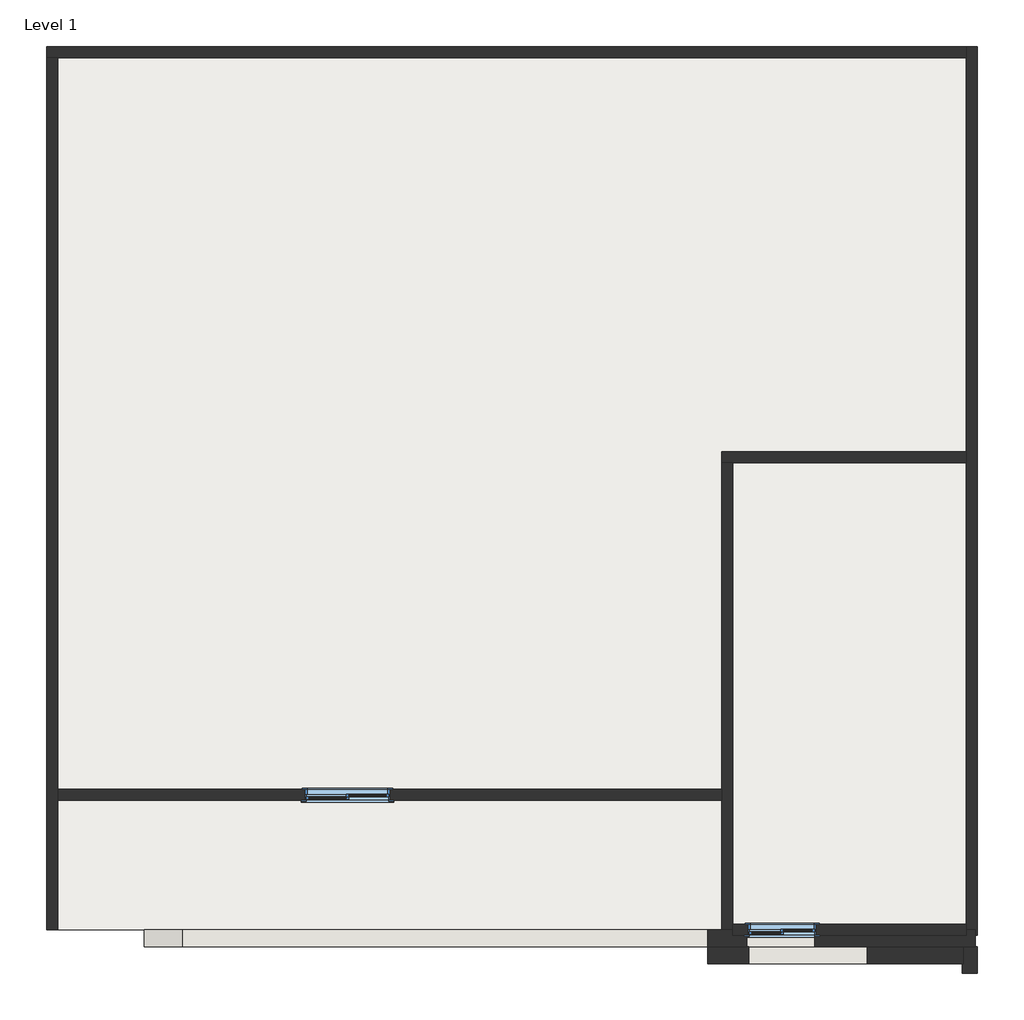
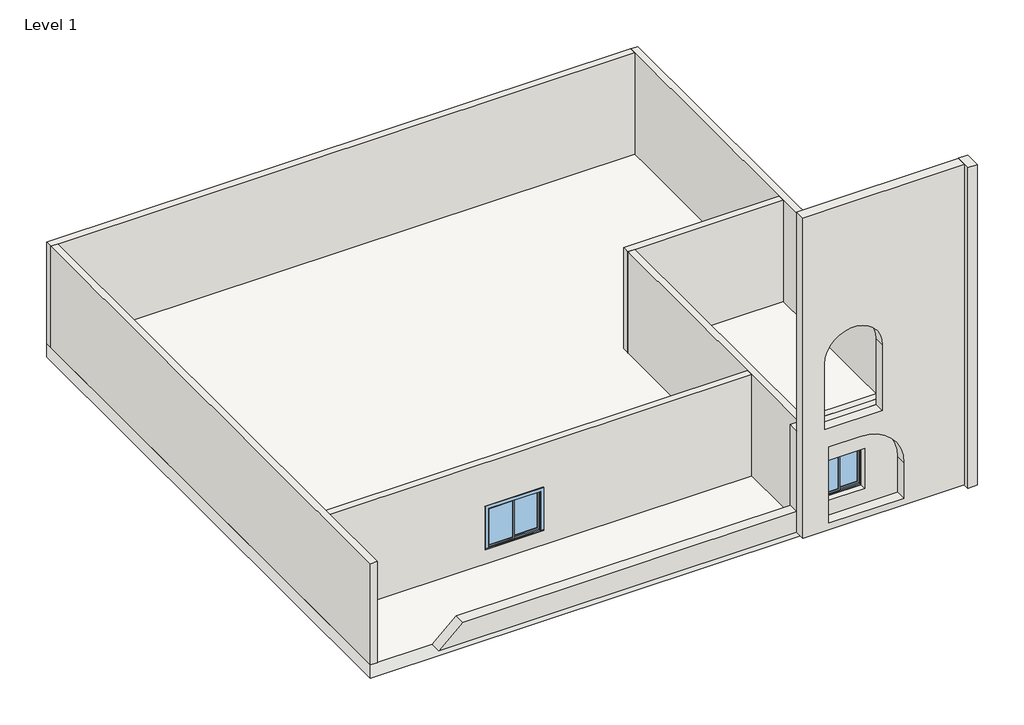
# One storey: 10 walls, 2 windows, 1 slab.
"""IFC4 building model written with IfcOpenShell, lengths in millimetres."""

from ifc_helpers import new_model, si_unit, frame, origin, place, context, project, spatial, polyline, outline, extrude, faceted_brep, transform, mapped, element, save
from components import walls_3_walls_3_95cfad7e, walls_4_walls_4_52940900, walls_6_walls_6_1b60e08d, window_deda82dd, window_c4d7a2b1

model = new_model("IFC4")

# Units and contexts
model_context = context("Model", 3, world=origin())
ifc_project = project(units=[si_unit("LENGTHUNIT", "METRE", prefix="MILLI")], contexts=[model_context])

# Site, building, storey
site = spatial("IfcSite", under=ifc_project)
building = spatial("IfcBuilding", under=site)
storey = spatial("IfcBuildingStorey", under=building, Name="Level 1", Elevation=3048.0)

# Slab
placement = place(None, origin())
element("IfcSlab", 1, ObjectType="Generic Floor - 400mm", at=placement, inside=storey, context=model_context, shape_type="SweptSolid", body=[
    extrude(outline(polyline([(-9031.8352527, 15360.4148445), (7778.3159626, 15360.4148445), (7778.3159626, -589.1851555), (-9031.8352527, -589.1851555), (-9031.8352527, 15360.4148445)])), frame((0.0, 0.0, 2648.0), z_axis=(0.0, 0.0, 1.0), x_axis=(1.0, 0.0, 0.0)), (0.0, 0.0, 1.0), 400.0),
])

# Walls
element("IfcWall", 2, ObjectType="Generic - 9\"", at=placement, inside=storey, context=model_context, shape_type="Brep", body=[
    faceted_brep([(-9031.8352527, 15160.4148445, 3048.0), (-8831.8352527, 15160.4148445, 3048.0), (7578.3159626, 15160.4148445, 3048.0), (7578.3159626, 15160.4148445, 6096.0), (-8831.8352527, 15160.4148445, 6096.0), (-9031.8352527, 15160.4148445, 6096.0), (-9031.8352527, 15360.4148445, 3048.0), (-9031.8352527, 15360.4148445, 6096.0), (7578.3159626, 15360.4148445, 6096.0), (7578.3159626, 15360.4148445, 3048.0)], [[[0, 1, 2, 3, 4, 5]], [[6, 7, 8, 9]], [[2, 1, 0, 6, 9]], [[5, 4, 3, 8, 7]], [[0, 5, 7, 6]], [[3, 2, 9, 8]]]),
])
element("IfcWall", 3, ObjectType="Generic - 9\"", at=placement, inside=storey, context=model_context, shape_type="Brep", body=[
    faceted_brep([(-8831.8352527, -589.1851555, 3048.0), (-8831.8352527, 1749.2148445, 3048.0), (-8831.8352527, 1949.2148445, 3048.0), (-8831.8352527, 15160.4148445, 3048.0), (-8831.8352527, 15160.4148445, 6096.0), (-8831.8352527, 1949.2148445, 6096.0), (-8831.8352527, 1749.2148445, 6096.0), (-8831.8352527, -589.1851555, 6096.0), (-9031.8352527, -589.1851555, 3048.0), (-9031.8352527, -589.1851555, 6096.0), (-9031.8352527, 15160.4148445, 6096.0), (-9031.8352527, 15160.4148445, 3048.0)], [[[0, 1, 2, 3, 4, 5, 6, 7]], [[8, 9, 10, 11]], [[3, 2, 1, 0, 8, 11]], [[7, 6, 5, 4, 10, 9]], [[0, 7, 9, 8]], [[4, 3, 11, 10]]]),
])
element("IfcWall", 4, ObjectType="Generic - 9\"", at=placement, inside=storey, context=model_context, shape_type="Brep", body=[
    faceted_brep([(7578.3159626, 15360.4148445, 3048.0), (7578.3159626, 15160.4148445, 3048.0), (7578.3159626, 8045.2148445, 3048.0), (7578.3159626, 7845.2148445, 3048.0), (7578.3159626, -489.1851555, 3048.0), (7578.3159626, -589.1851555, 3048.0), (7578.3159626, -689.1851555, 3048.0), (7578.3159626, -689.1851555, 6096.0), (7578.3159626, -489.1851555, 6096.0), (7578.3159626, 7845.2148445, 6096.0), (7578.3159626, 8045.2148445, 6096.0), (7578.3159626, 15160.4148445, 6096.0), (7578.3159626, 15360.4148445, 6096.0), (7778.3159626, 15360.4148445, 3048.0), (7778.3159626, 15360.4148445, 6096.0), (7778.3159626, -689.1851555, 6096.0), (7778.3159626, -689.1851555, 3048.0), (7778.3159626, -589.1851555, 3048.0), (7778.3159626, -489.1851555, 3048.0)], [[[0, 1, 2, 3, 4, 5, 6, 7, 8, 9, 10, 11, 12]], [[13, 14, 15, 16, 17, 18]], [[6, 5, 4, 3, 2, 1, 0, 13, 18, 17, 16]], [[12, 11, 10, 9, 8, 7, 15, 14]], [[0, 12, 14, 13]], [[7, 6, 16, 15]]]),
])
element("IfcWall", 5, ObjectType="Generic - 9\"", at=placement, inside=storey, context=model_context, shape_type="Brep", body=[
    faceted_brep([(3160.1647473, 7845.2148445, 3048.0), (3360.1647473, 7845.2148445, 3048.0), (7578.3159626, 7845.2148445, 3048.0), (7578.3159626, 7845.2148445, 6096.0), (3360.1647473, 7845.2148445, 6096.0), (3160.1647473, 7845.2148445, 6096.0), (3160.1647473, 8045.2148445, 3048.0), (3160.1647473, 8045.2148445, 6096.0), (7578.3159626, 8045.2148445, 6096.0), (7578.3159626, 8045.2148445, 3048.0)], [[[0, 1, 2, 3, 4, 5]], [[6, 7, 8, 9]], [[2, 1, 0, 6, 9]], [[5, 4, 3, 8, 7]], [[0, 5, 7, 6]], [[3, 2, 9, 8]]]),
])
element("IfcWall", 6, ObjectType="Generic - 9\"", at=placement, inside=storey, context=model_context, shape_type="Brep", body=[
    faceted_brep([(3360.1647473, -689.1851555, 3048.0), (3360.1647473, -489.1851555, 3048.0), (3360.1647473, 7845.2148445, 3048.0), (3360.1647473, 7845.2148445, 6096.0), (3360.1647473, -489.1851555, 6096.0), (3360.1647473, -689.1851555, 6096.0), (3160.1647473, -689.1851555, 3048.0), (3160.1647473, -689.1851555, 6096.0), (3160.1647473, 1749.2148445, 6096.0), (3160.1647473, 1949.2148445, 6096.0), (3160.1647473, 7845.2148445, 6096.0), (3160.1647473, 7845.2148445, 3048.0), (3160.1647473, 1949.2148445, 3048.0), (3160.1647473, 1749.2148445, 3048.0)], [[[0, 1, 2, 3, 4, 5]], [[6, 7, 8, 9, 10, 11, 12, 13]], [[2, 1, 0, 6, 13, 12, 11]], [[5, 4, 3, 10, 9, 8, 7]], [[3, 2, 11, 10]], [[0, 5, 7, 6]]]),
])
element("IfcWall", 7, ObjectType="Generic - 9\"", at=placement, inside=storey, context=model_context, shape_type="SweptSolid", body=[
    extrude(outline(polyline([(3048.0, 3160.1647473), (6096.0, 3160.1647473), (6096.0, -8831.8352527), (3048.0, -8831.8352527), (3048.0, 3160.1647473)]), holes=[polyline([(4724.4, -4359.8352527), (4724.4, -2835.8352527), (3505.2, -2835.8352527), (3505.2, -4359.8352527), (4724.4, -4359.8352527)])]), frame((0.0, 1749.2148445, 0.0), z_axis=(0.0, 1.0, 0.0), x_axis=(0.0, 0.0, 1.0)), (0.0, 0.0, 1.0), 200.0),
])
element("IfcWall", 8, ObjectType="Generic - 9\"", at=placement, inside=storey, context=model_context, shape_type="SweptSolid", body=[
    extrude(outline(polyline([(3048.0, 3360.1647473), (3048.0, 7578.3159626), (6096.0, 7578.3159626), (6096.0, 3360.1647473), (3048.0, 3360.1647473)]), holes=[polyline([(4906.7280725, 3641.1647473), (4906.7280725, 4860.3647473), (3687.5280725, 4860.3647473), (3687.5280725, 3641.1647473), (4906.7280725, 3641.1647473)])]), frame((0.0, -689.1851555, 0.0), z_axis=(0.0, 1.0, 0.0), x_axis=(0.0, 0.0, 1.0)), (0.0, 0.0, 1.0), 200.0),
])
walls_3_walls_3_shape = walls_3_walls_3_95cfad7e(model_context)
element("IfcWall", 9, ObjectType="Walls 3 : Walls 3", at=placement, inside=storey, context=model_context, shape_type="MappedRepresentation", body=[
    mapped(walls_3_walls_3_shape, transform((0.0, 0.0, 0.0), x_axis=(1.0, 0.0, 0.0), y_axis=(0.0, 1.0, 0.0), z_axis=(0.0, 0.0, 1.0))),
])
walls_4_walls_4_shape = walls_4_walls_4_52940900(model_context)
element("IfcWall", 10, ObjectType="Walls 4 : Walls 4", at=placement, inside=storey, context=model_context, shape_type="MappedRepresentation", body=[
    mapped(walls_4_walls_4_shape, transform((0.0, 0.0, 0.0), x_axis=(1.0, 0.0, 0.0), y_axis=(0.0, 1.0, 0.0), z_axis=(0.0, 0.0, 1.0))),
])
walls_6_walls_6_shape = walls_6_walls_6_1b60e08d(model_context)
element("IfcWall", 11, ObjectType="Walls 6 : Walls 6", at=placement, inside=storey, context=model_context, shape_type="MappedRepresentation", body=[
    mapped(walls_6_walls_6_shape, transform((0.0, 0.0, 0.0), x_axis=(1.0, 0.0, 0.0), y_axis=(0.0, 1.0, 0.0), z_axis=(0.0, 0.0, 1.0))),
])

# Windows
window_shape = window_deda82dd(model_context)
element("IfcWindow", 12, ObjectType="Slider with Trim : 48\" x 48\"", at=placement, inside=storey, context=model_context, shape_type="MappedRepresentation", body=[
    mapped(window_shape, transform((4250.7647473, -589.1851555, 2773.1280725), x_axis=(-1.0, 0.0, 0.0), y_axis=(0.0, -1.0, 0.0), z_axis=(0.0, 0.0, 1.0))),
])
window_2_shape = window_c4d7a2b1(model_context)
element("IfcWindow", 13, ObjectType="Slider with Trim : 60\" x 48\"", at=placement, inside=storey, context=model_context, shape_type="MappedRepresentation", body=[
    mapped(window_2_shape, transform((-3597.8352527, 1849.2148445, 2590.8), x_axis=(-1.0, 0.0, 0.0), y_axis=(0.0, -1.0, 0.0), z_axis=(0.0, 0.0, 1.0))),
])

save(model, "model.ifc")

# Revit data of these elements
# Type "Generic Floor - 400mm"
#   Function = 0
#   Layers, outside or top first: 1' - 3.74803" no material (function 1)
# Type "Generic - 9\""
#   Layers, outside or top first: 0' - 7.87402" no material (function 1)
# Type "Slider with Trim : 48\" x 48\""
#   Type Mark = "24"
#   Construction Type Id = "GSP4R"
#   Assembly Code = "B2020100"
#   Analytic Construction = "1/8 in Pilkington single glazing"
#   Visual Light Transmittance = 0.9
#   Solar Heat Gain Coefficient = 0.78
#   Heat Transfer Coefficient (U) = 3.6886 W/(m²·K)
#   Height = 4' - 0"
#   Default Sill Height = 3' - 0"
#   Trim Projection - Ext. = 0' - 0 3/4"
#   Trim Projection - Int. = 0' - 0 3/4"
#   Trim Width - Exterior = 0' - 3 1/2"
#   Trim Width - Interior = 0' - 3 1/2"
#   Width = 4' - 0"
#   Window Inset = 0' - 0 3/4"
#   Define Thermal Properties by = 1
#   Glass Pane Material = Glass
#   Sash Material = Sash
#   Trim Exterior Material = Trim
#   Trim Interior Material = Trim
#   Wall Closure = (empty or 0)
# Type "Slider with Trim : 60\" x 48\""
#   Type Mark = "22"
#   Construction Type Id = "GSP4R"
#   Assembly Code = "B2020100"
#   Analytic Construction = "1/8 in Pilkington single glazing"
#   Visual Light Transmittance = 0.9
#   Solar Heat Gain Coefficient = 0.78
#   Heat Transfer Coefficient (U) = 3.6886 W/(m²·K)
#   Height = 4' - 0"
#   Default Sill Height = 3' - 0"
#   Trim Projection - Ext. = 0' - 0 3/4"
#   Trim Projection - Int. = 0' - 0 3/4"
#   Trim Width - Exterior = 0' - 3 1/2"
#   Trim Width - Interior = 0' - 3 1/2"
#   Width = 5' - 0"
#   Window Inset = 0' - 0 3/4"
#   Define Thermal Properties by = 1
#   Glass Pane Material = Glass
#   Sash Material = Sash
#   Trim Exterior Material = Trim
#   Trim Interior Material = Trim
#   Wall Closure = (empty or 0)
# Element 1 (IfcSlab, "Generic Floor - 400mm")
#   built-in parameter 1001955 = 3.14159 (stored number, unit not read)
#   Height Offset From Level = 0' - 0"
#   Phase Created = New Construction
#   Materials on its faces: "Default Roof"
# Elements 2, 3, 4, 5, 6, 7, 8 (IfcWall, "Generic - 9\"")
#   Top Offset = 0' - 0"
#   Base Offset = 0' - 0"
#   Unconnected Height = 10' - 0"
#   wall height = 10' - 0"
#   Phase Created = New Construction
#   Base Constraint = Level 1
#   Materials on its faces: "Default Wall"
# Element 9 (IfcWall, "Walls 3 : Walls 3")
#   Phase Created = New Construction
#   Materials on its faces: "Default Wall"
# Element 10 (IfcWall, "Walls 4 : Walls 4")
#   Phase Created = New Construction
#   Materials on its faces: "Default Wall"
# Element 11 (IfcWall, "Walls 6 : Walls 6")
#   Phase Created = New Construction
#   Materials on its faces: "Default Wall"
# Element 12 (IfcWindow, "Slider with Trim : 48\" x 48\"")
#   Mark = "12"
#   Phase Created = New Construction
#   Materials on its faces: "Sash", "Trim", "Glass"
# Element 13 (IfcWindow, "Slider with Trim : 60\" x 48\"")
#   Mark = "8"
#   Phase Created = New Construction
#   Materials on its faces: "Sash", "Trim", "Glass"
# Materials
#   "Glass": class "Glass", colour RGB 218 227 224, transparency 0.85, Description = "Soda Lime Glass", Cost = 0
#   "Sash": class "Wood", colour RGB 136 99 55, transparency 0
#   "Trim": class "Wood", colour RGB 224 178 126, transparency 0
#   "Default Roof": colour RGB 80 80 80, transparency 0
#   "Default Wall": colour RGB 80 80 80, transparency 0
